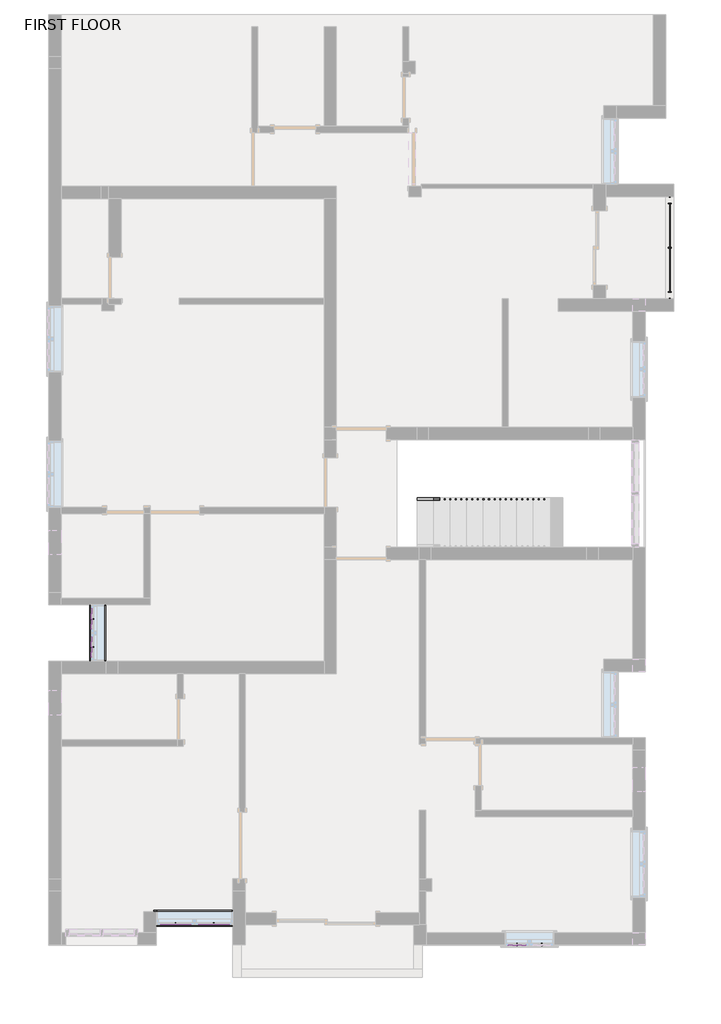
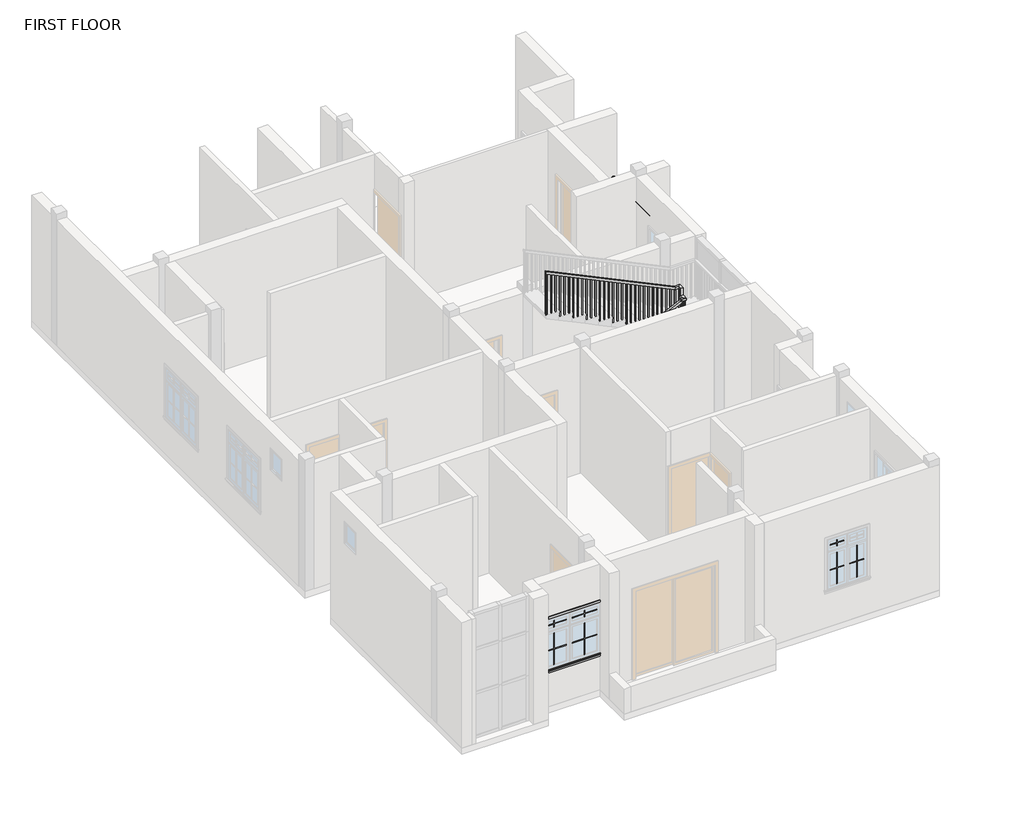
# One storey, part 5 of 6: 15 proxies, 2 railings.
"""IFC4 building model written with IfcOpenShell, lengths in millimetres."""

from ifc_helpers import new_model, si_unit, point, frame, origin, place, context, project, spatial, polyline, ellipse_curve, trimmed, outline, extrude, faceted_brep, transform, mapped, element, save
from ifc_brep_helpers import plane_surface, extruded_surface, advanced_brep
from components import muntin_pattern_2x2_muntin_pattern_2x2_a154cbfa, muntin_pattern_2x2_muntin_pattern_2x2_fbb866f2, muntin_pattern_2x2_muntin_pattern_2x2_1a5162a2, muntin_pattern_2x2_muntin_pattern_2x2_4af9dbf3, muntin_pattern_2x2_muntin_pattern_2x2_972acb6d, muntin_pattern_2x2_muntin_pattern_2x2_4879a4f3, muntin_pattern_2x2_muntin_pattern_2x2_d1c6e638, muntin_pattern_2x2_muntin_pattern_2x2_37b95fb2, muntin_pattern_2x2_muntin_pattern_2x2_604ffb00, trim_window_exterior_flat_with_sill_cb7cc766, trim_window_exterior_flat_with_sill_29d7a895, trim_window_interior_flat_picture_frame_9050e5f4, trim_window_interior_flat_picture_frame_56711e78

model = new_model("IFC4")

# Units and contexts
model_context = context("Model", 3, world=origin())
ifc_project = project(units=[si_unit("LENGTHUNIT", "METRE", prefix="MILLI")], contexts=[model_context])

# Site, building, storey
site = spatial("IfcSite", under=ifc_project)
building = spatial("IfcBuilding", under=site)
storey = spatial("IfcBuildingStorey", under=building, Name="FIRST FLOOR", Elevation=3200.4)

# Proxies
placement = place(None, origin())
muntin_pattern_2x2_muntin_pattern_2x2_shape = muntin_pattern_2x2_muntin_pattern_2x2_a154cbfa(model_context)
element("IfcBuildingElementProxy", 1, Name="Muntin Pattern_2x2 : Muntin Pattern_2x2", ObjectType="Muntin Pattern_2x2 : Muntin Pattern_2x2", at=placement, inside=storey, context=model_context, shape_type="MappedRepresentation", body=[
    mapped(muntin_pattern_2x2_muntin_pattern_2x2_shape, transform((-3731.5990981, -7428.8962413, 4184.65), x_axis=(-1.0, 0.0, 0.0), y_axis=(0.0, -1.0, 0.0), z_axis=(0.0, 0.0, 1.0))),
])
muntin_pattern_2x2_muntin_pattern_2x2_2_shape = muntin_pattern_2x2_muntin_pattern_2x2_fbb866f2(model_context)
element("IfcBuildingElementProxy", 2, Name="Muntin Pattern_2x2 : Muntin Pattern_2x2", ObjectType="Muntin Pattern_2x2 : Muntin Pattern_2x2", at=placement, inside=storey, context=model_context, shape_type="MappedRepresentation", body=[
    mapped(muntin_pattern_2x2_muntin_pattern_2x2_2_shape, transform((-4433.2740981, -7428.8962413, 4184.65), x_axis=(1.0, 0.0, 0.0), y_axis=(0.0, 1.0, 0.0), z_axis=(0.0, 0.0, 1.0))),
])
muntin_pattern_2x2_muntin_pattern_2x2_3_shape = muntin_pattern_2x2_muntin_pattern_2x2_1a5162a2(model_context)
element("IfcBuildingElementProxy", 3, Name="Muntin Pattern_2x2 : Muntin Pattern_2x2", ObjectType="Muntin Pattern_2x2 : Muntin Pattern_2x2", at=placement, inside=storey, context=model_context, shape_type="MappedRepresentation", body=[
    mapped(muntin_pattern_2x2_muntin_pattern_2x2_3_shape, transform((-4433.2740981, -7428.8962413, 5099.05), x_axis=(1.0, 0.0, 0.0), y_axis=(0.0, 1.0, 0.0), z_axis=(0.0, 0.0, 1.0))),
])
element("IfcBuildingElementProxy", 4, Name="Muntin Pattern_2x2 : Muntin Pattern_2x2", ObjectType="Muntin Pattern_2x2 : Muntin Pattern_2x2", at=placement, inside=storey, context=model_context, shape_type="MappedRepresentation", body=[
    mapped(muntin_pattern_2x2_muntin_pattern_2x2_3_shape, transform((-3731.5990981, -7428.8962413, 5099.05), x_axis=(1.0, 0.0, 0.0), y_axis=(0.0, 1.0, 0.0), z_axis=(0.0, 0.0, 1.0))),
])
muntin_pattern_2x2_muntin_pattern_2x2_4_shape = muntin_pattern_2x2_muntin_pattern_2x2_4af9dbf3(model_context)
element("IfcBuildingElementProxy", 5, Name="Muntin Pattern_2x2 : Muntin Pattern_2x2", ObjectType="Muntin Pattern_2x2 : Muntin Pattern_2x2", at=placement, inside=storey, context=model_context, shape_type="MappedRepresentation", body=[
    mapped(muntin_pattern_2x2_muntin_pattern_2x2_4_shape, transform((-5964.7636947, -2337.7837413, 4184.65), x_axis=(0.0, 1.0, 0.0), y_axis=(-1.0, 0.0, 0.0), z_axis=(0.0, 0.0, 1.0))),
])
muntin_pattern_2x2_muntin_pattern_2x2_5_shape = muntin_pattern_2x2_muntin_pattern_2x2_972acb6d(model_context)
element("IfcBuildingElementProxy", 6, Name="Muntin Pattern_2x2 : Muntin Pattern_2x2", ObjectType="Muntin Pattern_2x2 : Muntin Pattern_2x2", at=placement, inside=storey, context=model_context, shape_type="MappedRepresentation", body=[
    mapped(muntin_pattern_2x2_muntin_pattern_2x2_5_shape, transform((-5964.7636947, -1820.2587413, 4184.65), x_axis=(0.0, -1.0, 0.0), y_axis=(1.0, 0.0, 0.0), z_axis=(0.0, 0.0, 1.0))),
])
muntin_pattern_2x2_muntin_pattern_2x2_6_shape = muntin_pattern_2x2_muntin_pattern_2x2_4879a4f3(model_context)
element("IfcBuildingElementProxy", 7, Name="Muntin Pattern_2x2 : Muntin Pattern_2x2", ObjectType="Muntin Pattern_2x2 : Muntin Pattern_2x2", at=placement, inside=storey, context=model_context, shape_type="MappedRepresentation", body=[
    mapped(muntin_pattern_2x2_muntin_pattern_2x2_6_shape, transform((-5964.7636947, -1820.2587413, 5099.05), x_axis=(0.0, -1.0, 0.0), y_axis=(1.0, 0.0, 0.0), z_axis=(0.0, 0.0, 1.0))),
])
element("IfcBuildingElementProxy", 8, Name="Muntin Pattern_2x2 : Muntin Pattern_2x2", ObjectType="Muntin Pattern_2x2 : Muntin Pattern_2x2", at=placement, inside=storey, context=model_context, shape_type="MappedRepresentation", body=[
    mapped(muntin_pattern_2x2_muntin_pattern_2x2_6_shape, transform((-5964.7636947, -2337.7837413, 5099.05), x_axis=(0.0, -1.0, 0.0), y_axis=(1.0, 0.0, 0.0), z_axis=(0.0, 0.0, 1.0))),
])
muntin_pattern_2x2_muntin_pattern_2x2_7_shape = muntin_pattern_2x2_muntin_pattern_2x2_d1c6e638(model_context)
element("IfcBuildingElementProxy", 9, Name="Muntin Pattern_2x2 : Muntin Pattern_2x2", ObjectType="Muntin Pattern_2x2 : Muntin Pattern_2x2", at=placement, inside=storey, context=model_context, shape_type="MappedRepresentation", body=[
    mapped(muntin_pattern_2x2_muntin_pattern_2x2_7_shape, transform((2304.0759019, -7809.8962413, 4184.65), x_axis=(-1.0, 0.0, 0.0), y_axis=(0.0, -1.0, 0.0), z_axis=(0.0, 0.0, 1.0))),
])
muntin_pattern_2x2_muntin_pattern_2x2_8_shape = muntin_pattern_2x2_muntin_pattern_2x2_37b95fb2(model_context)
element("IfcBuildingElementProxy", 10, Name="Muntin Pattern_2x2 : Muntin Pattern_2x2", ObjectType="Muntin Pattern_2x2 : Muntin Pattern_2x2", at=placement, inside=storey, context=model_context, shape_type="MappedRepresentation", body=[
    mapped(muntin_pattern_2x2_muntin_pattern_2x2_8_shape, transform((1850.0509019, -7809.8962413, 4184.65), x_axis=(1.0, 0.0, 0.0), y_axis=(0.0, 1.0, 0.0), z_axis=(0.0, 0.0, 1.0))),
])
muntin_pattern_2x2_muntin_pattern_2x2_9_shape = muntin_pattern_2x2_muntin_pattern_2x2_604ffb00(model_context)
element("IfcBuildingElementProxy", 11, Name="Muntin Pattern_2x2 : Muntin Pattern_2x2", ObjectType="Muntin Pattern_2x2 : Muntin Pattern_2x2", at=placement, inside=storey, context=model_context, shape_type="MappedRepresentation", body=[
    mapped(muntin_pattern_2x2_muntin_pattern_2x2_9_shape, transform((1850.0509019, -7809.8962413, 5099.05), x_axis=(1.0, 0.0, 0.0), y_axis=(0.0, 1.0, 0.0), z_axis=(0.0, 0.0, 1.0))),
])
trim_window_exterior_flat_with_sill_shape = trim_window_exterior_flat_with_sill_cb7cc766(model_context)
element("IfcBuildingElementProxy", 12, Name="Trim-Window-Exterior-Flat : with Sill", ObjectType="Trim-Window-Exterior-Flat : with Sill", at=placement, inside=storey, context=model_context, shape_type="MappedRepresentation", body=[
    mapped(trim_window_exterior_flat_with_sill_shape, transform((-4082.4365981, -7438.4212413, 5334.0), x_axis=(1.0, 0.0, 0.0), y_axis=(0.0, 0.0, 1.0), z_axis=(0.0, -1.0, 0.0))),
])
trim_window_exterior_flat_with_sill_2_shape = trim_window_exterior_flat_with_sill_29d7a895(model_context)
element("IfcBuildingElementProxy", 13, Name="Trim-Window-Exterior-Flat : with Sill", ObjectType="Trim-Window-Exterior-Flat : with Sill", at=placement, inside=storey, context=model_context, shape_type="MappedRepresentation", body=[
    mapped(trim_window_exterior_flat_with_sill_2_shape, transform((-5974.2886947, -2079.0212413, 5334.0), x_axis=(0.0, -1.0, 0.0), y_axis=(0.0, 0.0, 1.0), z_axis=(-1.0, 0.0, 0.0))),
])
trim_window_interior_flat_picture_frame_shape = trim_window_interior_flat_picture_frame_9050e5f4(model_context)
element("IfcBuildingElementProxy", 14, Name="Trim-Window-Interior-Flat : Picture Frame", ObjectType="Trim-Window-Interior-Flat : Picture Frame", at=placement, inside=storey, context=model_context, shape_type="MappedRepresentation", body=[
    mapped(trim_window_interior_flat_picture_frame_shape, transform((-4082.4365981, -7209.8212413, 5334.0), x_axis=(-1.0, 0.0, 0.0), y_axis=(0.0, 0.0, 1.0), z_axis=(0.0, 1.0, 0.0))),
])
trim_window_interior_flat_picture_frame_2_shape = trim_window_interior_flat_picture_frame_56711e78(model_context)
element("IfcBuildingElementProxy", 15, Name="Trim-Window-Interior-Flat : Picture Frame", ObjectType="Trim-Window-Interior-Flat : Picture Frame", at=placement, inside=storey, context=model_context, shape_type="MappedRepresentation", body=[
    mapped(trim_window_interior_flat_picture_frame_2_shape, transform((-5745.6886947, -2079.0212413, 5334.0), x_axis=(0.0, 1.0, 0.0), y_axis=(0.0, 0.0, 1.0), z_axis=(1.0, 0.0, 0.0))),
])

# Railings
element("IfcRailing", 16, ObjectType="Glass Panel - Bottom Fill", at=placement, inside=storey, context=model_context, shape_type="SolidModel", body=[
    advanced_brep(
    [(4699.6134019, 5947.3787587, 4724.4), (4623.4134019, 5947.3787587, 4724.4), (4699.6134019, 4067.7787587, 4724.4), (4623.4134019, 4067.7787587, 4724.4)],
    [
        (0, 1, ellipse_curve(frame((4661.5134019, 5947.3787587, 4724.4), z_axis=(0.0, 1.0, 0.0), x_axis=(-1.0, 0.0, 0.0)), 38.1, 28.575)),
        (1, 0, ellipse_curve(frame((4661.5134019, 5947.3787587, 4724.4), z_axis=(0.0, 1.0, 0.0), x_axis=(-1.0, 0.0, 0.0)), 38.1, 28.575)),
        (2, 3, ellipse_curve(frame((4661.5134019, 4067.7787587, 4724.4), z_axis=(0.0, -1.0, 0.0), x_axis=(-1.0, 0.0, 0.0)), 38.1, 28.575)),
        (3, 2, ellipse_curve(frame((4661.5134019, 4067.7787587, 4724.4), z_axis=(0.0, -1.0, 0.0), x_axis=(-1.0, 0.0, 0.0)), 38.1, 28.575)),
        (0, 2),
        (3, 1),
    ],
    [
        plane_surface(frame((4661.5134019, 5947.3787587, 4724.4), z_axis=(0.0, 1.0, 0.0), x_axis=(0.0, 0.0, -1.0))),
        plane_surface(frame((4661.5134019, 4067.7787587, 4724.4), z_axis=(0.0, -1.0, 0.0), x_axis=(0.0, 0.0, -1.0))),
        extruded_surface(trimmed(ellipse_curve(frame((4661.5134019, 4067.7787587, 4724.4), z_axis=(0.0, 1.0, 0.0), x_axis=(-1.0, 0.0, 0.0)), 38.1, 28.575), [point((4699.6134019, 4067.7787587, 4724.4))], [point((4623.4134019, 4067.7787587, 4724.4))], True, "CARTESIAN"), (0.0, 1879.6, 0.0), 1879.6),
        extruded_surface(trimmed(ellipse_curve(frame((4661.5134019, 4067.7787587, 4724.4), z_axis=(0.0, 1.0, 0.0), x_axis=(-1.0, 0.0, 0.0)), 38.1, 28.575), [point((4623.4134019, 4067.7787587, 4724.4))], [point((4699.6134019, 4067.7787587, 4724.4))], True, "CARTESIAN"), (0.0, 1879.6, 0.0), 1879.6),
    ],
    [
        (0, [[1, 2]]),
        (1, [[3, 4]]),
        (2, [[-1, 5, -4, 6]]),
        (3, [[-2, -6, -3, -5]]),
    ],
),
    extrude(outline(polyline([(4648.8134019, 5947.3787587), (4674.2134019, 5947.3787587), (4674.2134019, 4067.7787587), (4648.8134019, 4067.7787587), (4648.8134019, 5947.3787587)])), frame((0.0, 0.0, 4610.1), z_axis=(0.0, 0.0, 1.0), x_axis=(1.0, 0.0, 0.0)), (0.0, 0.0, 1.0), 25.4),
    extrude(outline(polyline([(4648.8134019, 5947.3787587), (4674.2134019, 5947.3787587), (4674.2134019, 4067.7787587), (4648.8134019, 4067.7787587), (4648.8134019, 5947.3787587)])), frame((0.0, 0.0, 4508.5), z_axis=(0.0, 0.0, 1.0), x_axis=(1.0, 0.0, 0.0)), (0.0, 0.0, 1.0), 25.4),
    extrude(outline(polyline([(4636.1134019, 4201.1287587), (4686.9134019, 4201.1287587), (4686.9134019, 4188.4287587), (4636.1134019, 4188.4287587), (4636.1134019, 4201.1287587)])), frame((0.0, 0.0, 3810.0), z_axis=(0.0, 0.0, 1.0), x_axis=(1.0, 0.0, 0.0)), (0.0, 0.0, 1.0), 885.825),
    extrude(outline(polyline([(4668.0485589, 5007.5787587), (4668.0485589, 4194.7787587), (4661.6985589, 4194.7787587), (4661.6985589, 5007.5787587), (4668.0485589, 5007.5787587)])), frame((0.0, 0.0, 3911.6), z_axis=(0.0, 0.0, 1.0), x_axis=(1.0, 0.0, 0.0)), (0.0, 0.0, 1.0), 596.9),
    extrude(outline(polyline([(4636.1134019, 5013.9287587), (4686.9134019, 5013.9287587), (4686.9134019, 5001.2287587), (4636.1134019, 5001.2287587), (4636.1134019, 5013.9287587)])), frame((0.0, 0.0, 3810.0), z_axis=(0.0, 0.0, 1.0), x_axis=(1.0, 0.0, 0.0)), (0.0, 0.0, 1.0), 885.825),
    extrude(outline(polyline([(4668.0485589, 5820.3787587), (4668.0485589, 5007.5787587), (4661.6985589, 5007.5787587), (4661.6985589, 5820.3787587), (4668.0485589, 5820.3787587)])), frame((0.0, 0.0, 3911.6), z_axis=(0.0, 0.0, 1.0), x_axis=(1.0, 0.0, 0.0)), (0.0, 0.0, 1.0), 596.9),
    extrude(outline(polyline([(4636.1134019, 5826.7287587), (4686.9134019, 5826.7287587), (4686.9134019, 5814.0287587), (4636.1134019, 5814.0287587), (4636.1134019, 5826.7287587)])), frame((0.0, 0.0, 3810.0), z_axis=(0.0, 0.0, 1.0), x_axis=(1.0, 0.0, 0.0)), (0.0, 0.0, 1.0), 885.825),
    extrude(outline(polyline([(4651.9884019, 4080.4787587), (4671.0384019, 4080.4787587), (4671.0384019, 4061.4287587), (4651.9884019, 4061.4287587), (4651.9884019, 4080.4787587)])), frame((0.0, 0.0, 3810.0), z_axis=(0.0, 0.0, 1.0), x_axis=(1.0, 0.0, 0.0)), (0.0, 0.0, 1.0), 885.825),
    extrude(outline(polyline([(4651.9884019, 5953.7287587), (4671.0384019, 5953.7287587), (4671.0384019, 5934.6787587), (4651.9884019, 5934.6787587), (4651.9884019, 5953.7287587)])), frame((0.0, 0.0, 3810.0), z_axis=(0.0, 0.0, 1.0), x_axis=(1.0, 0.0, 0.0)), (0.0, 0.0, 1.0), 885.825),
])
element("IfcRailing", 17, ObjectType="Handrail - Rectangular", at=placement, inside=storey, context=model_context, shape_type="SolidModel", body=[
    faceted_brep([(13.3134019, 410.1787587, 4260.2727273), (13.3134019, 410.1787587, 4203.9834559), (13.3134019, 359.3787587, 4203.9834559), (13.3134019, 359.3787587, 4260.2727273), (2985.1134019, 410.1787587, 5678.6318182), (3035.9134019, 410.1787587, 5646.5880014), (3035.9134019, 359.3787587, 5646.5880014), (2985.1134019, 359.3787587, 5678.6318182), (2985.1134019, 410.1787587, 5715.0), (3035.9134019, 410.1787587, 5664.2), (3035.9134019, 359.3787587, 5664.2), (2985.1134019, 359.3787587, 5715.0), (3061.3134019, 410.1787587, 5715.0), (3061.3134019, 410.1787587, 5664.2), (3112.1134019, 359.3787587, 5664.2), (3112.1134019, 359.3787587, 5715.0), (3061.3134019, 486.3787587, 5715.0), (3061.3134019, 537.1787587, 5664.2), (3112.1134019, 537.1787587, 5664.2), (3112.1134019, 486.3787587, 5715.0), (3061.3134019, 486.3787587, 5896.8409091), (3061.3134019, 537.1787587, 5846.0409091), (3112.1134019, 537.1787587, 5846.0409091), (3112.1134019, 486.3787587, 5896.8409091), (3061.3134019, 562.5787587, 5896.8409091), (3061.3134019, 562.5787587, 5846.0409091), (3112.1134019, 613.3787587, 5846.0409091), (3112.1134019, 613.3787587, 5896.8409091), (2985.1134019, 562.5787587, 5896.8409091), (2973.6120715, 562.5787587, 5846.0409091), (2973.6120715, 613.3787587, 5846.0409091), (2985.1134019, 613.3787587, 5896.8409091), (13.3134019, 562.5787587, 7315.2), (13.3134019, 613.3787587, 7315.2), (13.3134019, 613.3787587, 7258.9107287), (13.3134019, 562.5787587, 7258.9107287)], [[[0, 1, 2, 3]], [[1, 0, 4, 5]], [[2, 1, 5, 6]], [[3, 2, 6, 7]], [[0, 3, 7, 4]], [[5, 4, 8, 9]], [[6, 5, 9, 10]], [[7, 6, 10, 11]], [[4, 7, 11, 8]], [[9, 8, 12, 13]], [[10, 9, 13, 14]], [[11, 10, 14, 15]], [[8, 11, 15, 12]], [[13, 12, 16, 17]], [[14, 13, 17, 18]], [[15, 14, 18, 19]], [[12, 15, 19, 16]], [[17, 16, 20, 21]], [[18, 17, 21, 22]], [[19, 18, 22, 23]], [[16, 19, 23, 20]], [[21, 20, 24, 25]], [[22, 21, 25, 26]], [[23, 22, 26, 27]], [[20, 23, 27, 24]], [[25, 24, 28, 29]], [[26, 25, 29, 30]], [[27, 26, 30, 31]], [[24, 27, 31, 28]], [[32, 33, 34, 35]], [[29, 28, 32, 35]], [[30, 29, 35, 34]], [[31, 30, 34, 33]], [[28, 31, 33, 32]]]),
    extrude(outline(polyline([(7251.3340241, 29.1884019), (6255.3272727, 29.1884019), (6255.3272727, 48.2384019), (7242.2419787, 48.2384019), (7251.3340241, 29.1884019)])), frame((0.0, 578.4537587, 0.0), z_axis=(0.0, 1.0, 0.0), x_axis=(0.0, 0.0, 1.0)), (0.0, 0.0, 1.0), 19.05),
    extrude(outline(polyline([(7202.843115, 130.7884019), (6255.3272727, 130.7884019), (6255.3272727, 149.8384019), (7193.7510696, 149.8384019), (7202.843115, 130.7884019)])), frame((0.0, 578.4537587, 0.0), z_axis=(0.0, 1.0, 0.0), x_axis=(0.0, 0.0, 1.0)), (0.0, 0.0, 1.0), 19.05),
    extrude(outline(polyline([(7154.3522059, 232.3884019), (6255.3272727, 232.3884019), (6255.3272727, 251.4384019), (7145.2601605, 251.4384019), (7154.3522059, 232.3884019)])), frame((0.0, 578.4537587, 0.0), z_axis=(0.0, 1.0, 0.0), x_axis=(0.0, 0.0, 1.0)), (0.0, 0.0, 1.0), 19.05),
    extrude(outline(polyline([(7105.8612969, 333.9884019), (6109.8545455, 333.9884019), (6109.8545455, 353.0384019), (7096.7692514, 353.0384019), (7105.8612969, 333.9884019)])), frame((0.0, 578.4537587, 0.0), z_axis=(0.0, 1.0, 0.0), x_axis=(0.0, 0.0, 1.0)), (0.0, 0.0, 1.0), 19.05),
    extrude(outline(polyline([(7057.3703878, 435.5884019), (6109.8545455, 435.5884019), (6109.8545455, 454.6384019), (7048.2783423, 454.6384019), (7057.3703878, 435.5884019)])), frame((0.0, 578.4537587, 0.0), z_axis=(0.0, 1.0, 0.0), x_axis=(0.0, 0.0, 1.0)), (0.0, 0.0, 1.0), 19.05),
    extrude(outline(polyline([(7008.8794787, 537.1884019), (6109.8545455, 537.1884019), (6109.8545455, 556.2384019), (6999.7874332, 556.2384019), (7008.8794787, 537.1884019)])), frame((0.0, 578.4537587, 0.0), z_axis=(0.0, 1.0, 0.0), x_axis=(0.0, 0.0, 1.0)), (0.0, 0.0, 1.0), 19.05),
    extrude(outline(polyline([(6960.3885696, 638.7884019), (5964.3818182, 638.7884019), (5964.3818182, 657.8384019), (6951.2965241, 657.8384019), (6960.3885696, 638.7884019)])), frame((0.0, 578.4537587, 0.0), z_axis=(0.0, 1.0, 0.0), x_axis=(0.0, 0.0, 1.0)), (0.0, 0.0, 1.0), 19.05),
    extrude(outline(polyline([(6911.8976605, 740.3884019), (5964.3818182, 740.3884019), (5964.3818182, 759.4384019), (6902.805615, 759.4384019), (6911.8976605, 740.3884019)])), frame((0.0, 578.4537587, 0.0), z_axis=(0.0, 1.0, 0.0), x_axis=(0.0, 0.0, 1.0)), (0.0, 0.0, 1.0), 19.05),
    extrude(outline(polyline([(6863.4067514, 841.9884019), (5964.3818182, 841.9884019), (5964.3818182, 861.0384019), (6854.3147059, 861.0384019), (6863.4067514, 841.9884019)])), frame((0.0, 578.4537587, 0.0), z_axis=(0.0, 1.0, 0.0), x_axis=(0.0, 0.0, 1.0)), (0.0, 0.0, 1.0), 19.05),
    extrude(outline(polyline([(6814.9158423, 943.5884019), (5818.9090909, 943.5884019), (5818.9090909, 962.6384019), (6805.8237969, 962.6384019), (6814.9158423, 943.5884019)])), frame((0.0, 578.4537587, 0.0), z_axis=(0.0, 1.0, 0.0), x_axis=(0.0, 0.0, 1.0)), (0.0, 0.0, 1.0), 19.05),
    extrude(outline(polyline([(6766.4249332, 1045.1884019), (5818.9090909, 1045.1884019), (5818.9090909, 1064.2384019), (6757.3328878, 1064.2384019), (6766.4249332, 1045.1884019)])), frame((0.0, 578.4537587, 0.0), z_axis=(0.0, 1.0, 0.0), x_axis=(0.0, 0.0, 1.0)), (0.0, 0.0, 1.0), 19.05),
    extrude(outline(polyline([(6717.9340241, 1146.7884019), (5818.9090909, 1146.7884019), (5818.9090909, 1165.8384019), (6708.8419787, 1165.8384019), (6717.9340241, 1146.7884019)])), frame((0.0, 578.4537587, 0.0), z_axis=(0.0, 1.0, 0.0), x_axis=(0.0, 0.0, 1.0)), (0.0, 0.0, 1.0), 19.05),
    extrude(outline(polyline([(6669.443115, 1248.3884019), (5673.4363636, 1248.3884019), (5673.4363636, 1267.4384019), (6660.3510696, 1267.4384019), (6669.443115, 1248.3884019)])), frame((0.0, 578.4537587, 0.0), z_axis=(0.0, 1.0, 0.0), x_axis=(0.0, 0.0, 1.0)), (0.0, 0.0, 1.0), 19.05),
    extrude(outline(polyline([(6620.9522059, 1349.9884019), (5673.4363636, 1349.9884019), (5673.4363636, 1369.0384019), (6611.8601605, 1369.0384019), (6620.9522059, 1349.9884019)])), frame((0.0, 578.4537587, 0.0), z_axis=(0.0, 1.0, 0.0), x_axis=(0.0, 0.0, 1.0)), (0.0, 0.0, 1.0), 19.05),
    extrude(outline(polyline([(6572.4612969, 1451.5884019), (5673.4363636, 1451.5884019), (5673.4363636, 1470.6384019), (6563.3692514, 1470.6384019), (6572.4612969, 1451.5884019)])), frame((0.0, 578.4537587, 0.0), z_axis=(0.0, 1.0, 0.0), x_axis=(0.0, 0.0, 1.0)), (0.0, 0.0, 1.0), 19.05),
    extrude(outline(polyline([(6523.9703878, 1553.1884019), (5527.9636364, 1553.1884019), (5527.9636364, 1572.2384019), (6514.8783423, 1572.2384019), (6523.9703878, 1553.1884019)])), frame((0.0, 578.4537587, 0.0), z_axis=(0.0, 1.0, 0.0), x_axis=(0.0, 0.0, 1.0)), (0.0, 0.0, 1.0), 19.05),
    extrude(outline(polyline([(6475.4794787, 1654.7884019), (5527.9636364, 1654.7884019), (5527.9636364, 1673.8384019), (6466.3874332, 1673.8384019), (6475.4794787, 1654.7884019)])), frame((0.0, 578.4537587, 0.0), z_axis=(0.0, 1.0, 0.0), x_axis=(0.0, 0.0, 1.0)), (0.0, 0.0, 1.0), 19.05),
    extrude(outline(polyline([(6426.9885696, 1756.3884019), (5527.9636364, 1756.3884019), (5527.9636364, 1775.4384019), (6417.8965241, 1775.4384019), (6426.9885696, 1756.3884019)])), frame((0.0, 578.4537587, 0.0), z_axis=(0.0, 1.0, 0.0), x_axis=(0.0, 0.0, 1.0)), (0.0, 0.0, 1.0), 19.05),
    extrude(outline(polyline([(6378.4976605, 1857.9884019), (5382.4909091, 1857.9884019), (5382.4909091, 1877.0384019), (6369.405615, 1877.0384019), (6378.4976605, 1857.9884019)])), frame((0.0, 578.4537587, 0.0), z_axis=(0.0, 1.0, 0.0), x_axis=(0.0, 0.0, 1.0)), (0.0, 0.0, 1.0), 19.05),
    extrude(outline(polyline([(6330.0067514, 1959.5884019), (5382.4909091, 1959.5884019), (5382.4909091, 1978.6384019), (6320.9147059, 1978.6384019), (6330.0067514, 1959.5884019)])), frame((0.0, 578.4537587, 0.0), z_axis=(0.0, 1.0, 0.0), x_axis=(0.0, 0.0, 1.0)), (0.0, 0.0, 1.0), 19.05),
    extrude(outline(polyline([(6281.5158423, 2061.1884019), (5382.4909091, 2061.1884019), (5382.4909091, 2080.2384019), (6272.4237969, 2080.2384019), (6281.5158423, 2061.1884019)])), frame((0.0, 578.4537587, 0.0), z_axis=(0.0, 1.0, 0.0), x_axis=(0.0, 0.0, 1.0)), (0.0, 0.0, 1.0), 19.05),
    extrude(outline(polyline([(6233.0249332, 2162.7884019), (5237.0181818, 2162.7884019), (5237.0181818, 2181.8384019), (6223.9328878, 2181.8384019), (6233.0249332, 2162.7884019)])), frame((0.0, 578.4537587, 0.0), z_axis=(0.0, 1.0, 0.0), x_axis=(0.0, 0.0, 1.0)), (0.0, 0.0, 1.0), 19.05),
    extrude(outline(polyline([(6184.5340241, 2264.3884019), (5237.0181818, 2264.3884019), (5237.0181818, 2283.4384019), (6175.4419787, 2283.4384019), (6184.5340241, 2264.3884019)])), frame((0.0, 578.4537587, 0.0), z_axis=(0.0, 1.0, 0.0), x_axis=(0.0, 0.0, 1.0)), (0.0, 0.0, 1.0), 19.05),
    extrude(outline(polyline([(6136.043115, 2365.9884019), (5237.0181818, 2365.9884019), (5237.0181818, 2385.0384019), (6126.9510696, 2385.0384019), (6136.043115, 2365.9884019)])), frame((0.0, 578.4537587, 0.0), z_axis=(0.0, 1.0, 0.0), x_axis=(0.0, 0.0, 1.0)), (0.0, 0.0, 1.0), 19.05),
    extrude(outline(polyline([(6087.5522059, 2467.5884019), (5091.5454545, 2467.5884019), (5091.5454545, 2486.6384019), (6078.4601605, 2486.6384019), (6087.5522059, 2467.5884019)])), frame((0.0, 578.4537587, 0.0), z_axis=(0.0, 1.0, 0.0), x_axis=(0.0, 0.0, 1.0)), (0.0, 0.0, 1.0), 19.05),
    extrude(outline(polyline([(6039.0612969, 2569.1884019), (5091.5454545, 2569.1884019), (5091.5454545, 2588.2384019), (6029.9692514, 2588.2384019), (6039.0612969, 2569.1884019)])), frame((0.0, 578.4537587, 0.0), z_axis=(0.0, 1.0, 0.0), x_axis=(0.0, 0.0, 1.0)), (0.0, 0.0, 1.0), 19.05),
    extrude(outline(polyline([(5990.5703878, 2670.7884019), (5091.5454545, 2670.7884019), (5091.5454545, 2689.8384019), (5981.4783423, 2689.8384019), (5990.5703878, 2670.7884019)])), frame((0.0, 578.4537587, 0.0), z_axis=(0.0, 1.0, 0.0), x_axis=(0.0, 0.0, 1.0)), (0.0, 0.0, 1.0), 19.05),
    extrude(outline(polyline([(5942.0794787, 2772.3884019), (4946.0727273, 2772.3884019), (4946.0727273, 2791.4384019), (5932.9874332, 2791.4384019), (5942.0794787, 2772.3884019)])), frame((0.0, 578.4537587, 0.0), z_axis=(0.0, 1.0, 0.0), x_axis=(0.0, 0.0, 1.0)), (0.0, 0.0, 1.0), 19.05),
    extrude(outline(polyline([(5893.5885696, 2873.9884019), (4946.0727273, 2873.9884019), (4946.0727273, 2893.0384019), (5884.4965241, 2893.0384019), (5893.5885696, 2873.9884019)])), frame((0.0, 578.4537587, 0.0), z_axis=(0.0, 1.0, 0.0), x_axis=(0.0, 0.0, 1.0)), (0.0, 0.0, 1.0), 19.05),
    extrude(outline(polyline([(5845.0976605, 2975.5884019), (4946.0727273, 2975.5884019), (4946.0727273, 2994.6384019), (5836.005615, 2994.6384019), (5845.0976605, 2975.5884019)])), frame((0.0, 578.4537587, 0.0), z_axis=(0.0, 1.0, 0.0), x_axis=(0.0, 0.0, 1.0)), (0.0, 0.0, 1.0), 19.05),
    extrude(outline(polyline([(3077.1884019, 476.8537587), (3077.1884019, 495.9037587), (3096.2384019, 495.9037587), (3096.2384019, 476.8537587), (3077.1884019, 476.8537587)])), frame((0.0, 0.0, 4800.6), z_axis=(0.0, 0.0, 1.0), x_axis=(1.0, 0.0, 0.0)), (0.0, 0.0, 1.0), 863.6),
    extrude(outline(polyline([(3051.7884019, 394.3037587), (3070.8384019, 394.3037587), (3070.8384019, 375.2537587), (3051.7884019, 375.2537587), (3051.7884019, 394.3037587)])), frame((0.0, 0.0, 4800.6), z_axis=(0.0, 0.0, 1.0), x_axis=(1.0, 0.0, 0.0)), (0.0, 0.0, 1.0), 863.6),
    extrude(outline(polyline([(5605.6737969, 2950.1884019), (4655.1272727, 2950.1884019), (4655.1272727, 2969.2384019), (5614.7658423, 2969.2384019), (5605.6737969, 2950.1884019)])), frame((0.0, 375.2537587, 0.0), z_axis=(0.0, 1.0, 0.0), x_axis=(0.0, 0.0, 1.0)), (0.0, 0.0, 1.0), 19.05),
    extrude(outline(polyline([(5557.1828878, 2848.5884019), (4655.1272727, 2848.5884019), (4655.1272727, 2867.6384019), (5566.2749332, 2867.6384019), (5557.1828878, 2848.5884019)])), frame((0.0, 375.2537587, 0.0), z_axis=(0.0, 1.0, 0.0), x_axis=(0.0, 0.0, 1.0)), (0.0, 0.0, 1.0), 19.05),
    extrude(outline(polyline([(5508.6919787, 2746.9884019), (4655.1272727, 2746.9884019), (4655.1272727, 2766.0384019), (5517.7840241, 2766.0384019), (5508.6919787, 2746.9884019)])), frame((0.0, 375.2537587, 0.0), z_axis=(0.0, 1.0, 0.0), x_axis=(0.0, 0.0, 1.0)), (0.0, 0.0, 1.0), 19.05),
    extrude(outline(polyline([(5460.2010696, 2645.3884019), (4509.6545455, 2645.3884019), (4509.6545455, 2664.4384019), (5469.293115, 2664.4384019), (5460.2010696, 2645.3884019)])), frame((0.0, 375.2537587, 0.0), z_axis=(0.0, 1.0, 0.0), x_axis=(0.0, 0.0, 1.0)), (0.0, 0.0, 1.0), 19.05),
    extrude(outline(polyline([(5411.7101605, 2543.7884019), (4509.6545455, 2543.7884019), (4509.6545455, 2562.8384019), (5420.8022059, 2562.8384019), (5411.7101605, 2543.7884019)])), frame((0.0, 375.2537587, 0.0), z_axis=(0.0, 1.0, 0.0), x_axis=(0.0, 0.0, 1.0)), (0.0, 0.0, 1.0), 19.05),
    extrude(outline(polyline([(5363.2192514, 2442.1884019), (4509.6545455, 2442.1884019), (4509.6545455, 2461.2384019), (5372.3112969, 2461.2384019), (5363.2192514, 2442.1884019)])), frame((0.0, 375.2537587, 0.0), z_axis=(0.0, 1.0, 0.0), x_axis=(0.0, 0.0, 1.0)), (0.0, 0.0, 1.0), 19.05),
    extrude(outline(polyline([(5314.7283423, 2340.5884019), (4364.1818182, 2340.5884019), (4364.1818182, 2359.6384019), (5323.8203878, 2359.6384019), (5314.7283423, 2340.5884019)])), frame((0.0, 375.2537587, 0.0), z_axis=(0.0, 1.0, 0.0), x_axis=(0.0, 0.0, 1.0)), (0.0, 0.0, 1.0), 19.05),
    extrude(outline(polyline([(5266.2374332, 2238.9884019), (4364.1818182, 2238.9884019), (4364.1818182, 2258.0384019), (5275.3294787, 2258.0384019), (5266.2374332, 2238.9884019)])), frame((0.0, 375.2537587, 0.0), z_axis=(0.0, 1.0, 0.0), x_axis=(0.0, 0.0, 1.0)), (0.0, 0.0, 1.0), 19.05),
    extrude(outline(polyline([(5217.7465241, 2137.3884019), (4364.1818182, 2137.3884019), (4364.1818182, 2156.4384019), (5226.8385696, 2156.4384019), (5217.7465241, 2137.3884019)])), frame((0.0, 375.2537587, 0.0), z_axis=(0.0, 1.0, 0.0), x_axis=(0.0, 0.0, 1.0)), (0.0, 0.0, 1.0), 19.05),
    extrude(outline(polyline([(5169.255615, 2035.7884019), (4218.7090909, 2035.7884019), (4218.7090909, 2054.8384019), (5178.3476605, 2054.8384019), (5169.255615, 2035.7884019)])), frame((0.0, 375.2537587, 0.0), z_axis=(0.0, 1.0, 0.0), x_axis=(0.0, 0.0, 1.0)), (0.0, 0.0, 1.0), 19.05),
    extrude(outline(polyline([(5120.7647059, 1934.1884019), (4218.7090909, 1934.1884019), (4218.7090909, 1953.2384019), (5129.8567514, 1953.2384019), (5120.7647059, 1934.1884019)])), frame((0.0, 375.2537587, 0.0), z_axis=(0.0, 1.0, 0.0), x_axis=(0.0, 0.0, 1.0)), (0.0, 0.0, 1.0), 19.05),
    extrude(outline(polyline([(5072.2737969, 1832.5884019), (4218.7090909, 1832.5884019), (4218.7090909, 1851.6384019), (5081.3658423, 1851.6384019), (5072.2737969, 1832.5884019)])), frame((0.0, 375.2537587, 0.0), z_axis=(0.0, 1.0, 0.0), x_axis=(0.0, 0.0, 1.0)), (0.0, 0.0, 1.0), 19.05),
    extrude(outline(polyline([(5023.7828878, 1730.9884019), (4073.2363636, 1730.9884019), (4073.2363636, 1750.0384019), (5032.8749332, 1750.0384019), (5023.7828878, 1730.9884019)])), frame((0.0, 375.2537587, 0.0), z_axis=(0.0, 1.0, 0.0), x_axis=(0.0, 0.0, 1.0)), (0.0, 0.0, 1.0), 19.05),
    extrude(outline(polyline([(4975.2919787, 1629.3884019), (4073.2363636, 1629.3884019), (4073.2363636, 1648.4384019), (4984.3840241, 1648.4384019), (4975.2919787, 1629.3884019)])), frame((0.0, 375.2537587, 0.0), z_axis=(0.0, 1.0, 0.0), x_axis=(0.0, 0.0, 1.0)), (0.0, 0.0, 1.0), 19.05),
    extrude(outline(polyline([(4926.8010696, 1527.7884019), (4073.2363636, 1527.7884019), (4073.2363636, 1546.8384019), (4935.893115, 1546.8384019), (4926.8010696, 1527.7884019)])), frame((0.0, 375.2537587, 0.0), z_axis=(0.0, 1.0, 0.0), x_axis=(0.0, 0.0, 1.0)), (0.0, 0.0, 1.0), 19.05),
    extrude(outline(polyline([(4878.3101605, 1426.1884019), (3927.7636364, 1426.1884019), (3927.7636364, 1445.2384019), (4887.4022059, 1445.2384019), (4878.3101605, 1426.1884019)])), frame((0.0, 375.2537587, 0.0), z_axis=(0.0, 1.0, 0.0), x_axis=(0.0, 0.0, 1.0)), (0.0, 0.0, 1.0), 19.05),
    extrude(outline(polyline([(4829.8192514, 1324.5884019), (3927.7636364, 1324.5884019), (3927.7636364, 1343.6384019), (4838.9112969, 1343.6384019), (4829.8192514, 1324.5884019)])), frame((0.0, 375.2537587, 0.0), z_axis=(0.0, 1.0, 0.0), x_axis=(0.0, 0.0, 1.0)), (0.0, 0.0, 1.0), 19.05),
    extrude(outline(polyline([(4781.3283423, 1222.9884019), (3927.7636364, 1222.9884019), (3927.7636364, 1242.0384019), (4790.4203878, 1242.0384019), (4781.3283423, 1222.9884019)])), frame((0.0, 375.2537587, 0.0), z_axis=(0.0, 1.0, 0.0), x_axis=(0.0, 0.0, 1.0)), (0.0, 0.0, 1.0), 19.05),
    extrude(outline(polyline([(4732.8374332, 1121.3884019), (3782.2909091, 1121.3884019), (3782.2909091, 1140.4384019), (4741.9294787, 1140.4384019), (4732.8374332, 1121.3884019)])), frame((0.0, 375.2537587, 0.0), z_axis=(0.0, 1.0, 0.0), x_axis=(0.0, 0.0, 1.0)), (0.0, 0.0, 1.0), 19.05),
    extrude(outline(polyline([(4684.3465241, 1019.7884019), (3782.2909091, 1019.7884019), (3782.2909091, 1038.8384019), (4693.4385696, 1038.8384019), (4684.3465241, 1019.7884019)])), frame((0.0, 375.2537587, 0.0), z_axis=(0.0, 1.0, 0.0), x_axis=(0.0, 0.0, 1.0)), (0.0, 0.0, 1.0), 19.05),
    extrude(outline(polyline([(4635.855615, 918.1884019), (3782.2909091, 918.1884019), (3782.2909091, 937.2384019), (4644.9476605, 937.2384019), (4635.855615, 918.1884019)])), frame((0.0, 375.2537587, 0.0), z_axis=(0.0, 1.0, 0.0), x_axis=(0.0, 0.0, 1.0)), (0.0, 0.0, 1.0), 19.05),
    extrude(outline(polyline([(4587.3647059, 816.5884019), (3636.8181818, 816.5884019), (3636.8181818, 835.6384019), (4596.4567514, 835.6384019), (4587.3647059, 816.5884019)])), frame((0.0, 375.2537587, 0.0), z_axis=(0.0, 1.0, 0.0), x_axis=(0.0, 0.0, 1.0)), (0.0, 0.0, 1.0), 19.05),
    extrude(outline(polyline([(4538.8737969, 714.9884019), (3636.8181818, 714.9884019), (3636.8181818, 734.0384019), (4547.9658423, 734.0384019), (4538.8737969, 714.9884019)])), frame((0.0, 375.2537587, 0.0), z_axis=(0.0, 1.0, 0.0), x_axis=(0.0, 0.0, 1.0)), (0.0, 0.0, 1.0), 19.05),
    extrude(outline(polyline([(4490.3828878, 613.3884019), (3636.8181818, 613.3884019), (3636.8181818, 632.4384019), (4499.4749332, 632.4384019), (4490.3828878, 613.3884019)])), frame((0.0, 375.2537587, 0.0), z_axis=(0.0, 1.0, 0.0), x_axis=(0.0, 0.0, 1.0)), (0.0, 0.0, 1.0), 19.05),
    extrude(outline(polyline([(4441.8919787, 511.7884019), (3491.3454545, 511.7884019), (3491.3454545, 530.8384019), (4450.9840241, 530.8384019), (4441.8919787, 511.7884019)])), frame((0.0, 375.2537587, 0.0), z_axis=(0.0, 1.0, 0.0), x_axis=(0.0, 0.0, 1.0)), (0.0, 0.0, 1.0), 19.05),
    extrude(outline(polyline([(4393.4010696, 410.1884019), (3491.3454545, 410.1884019), (3491.3454545, 429.2384019), (4402.493115, 429.2384019), (4393.4010696, 410.1884019)])), frame((0.0, 375.2537587, 0.0), z_axis=(0.0, 1.0, 0.0), x_axis=(0.0, 0.0, 1.0)), (0.0, 0.0, 1.0), 19.05),
    extrude(outline(polyline([(4344.9101605, 308.5884019), (3491.3454545, 308.5884019), (3491.3454545, 327.6384019), (4354.0022059, 327.6384019), (4344.9101605, 308.5884019)])), frame((0.0, 375.2537587, 0.0), z_axis=(0.0, 1.0, 0.0), x_axis=(0.0, 0.0, 1.0)), (0.0, 0.0, 1.0), 19.05),
    extrude(outline(polyline([(4296.4192514, 206.9884019), (3345.8727273, 206.9884019), (3345.8727273, 226.0384019), (4305.5112969, 226.0384019), (4296.4192514, 206.9884019)])), frame((0.0, 375.2537587, 0.0), z_axis=(0.0, 1.0, 0.0), x_axis=(0.0, 0.0, 1.0)), (0.0, 0.0, 1.0), 19.05),
    extrude(outline(polyline([(4247.9283423, 105.3884019), (3345.8727273, 105.3884019), (3345.8727273, 124.4384019), (4257.0203878, 124.4384019), (4247.9283423, 105.3884019)])), frame((0.0, 375.2537587, 0.0), z_axis=(0.0, 1.0, 0.0), x_axis=(0.0, 0.0, 1.0)), (0.0, 0.0, 1.0), 19.05),
    extrude(outline(polyline([(3077.1884019, 578.4537587), (3077.1884019, 597.5037587), (3096.2384019, 597.5037587), (3096.2384019, 578.4537587), (3077.1884019, 578.4537587)])), frame((0.0, 0.0, 4800.6), z_axis=(0.0, 0.0, 1.0), x_axis=(1.0, 0.0, 0.0)), (0.0, 0.0, 1.0), 1045.4409091),
    extrude(outline(polyline([(3077.1884019, 394.3037587), (3096.2384019, 394.3037587), (3096.2384019, 375.2537587), (3077.1884019, 375.2537587), (3077.1884019, 394.3037587)])), frame((0.0, 0.0, 4800.6), z_axis=(0.0, 0.0, 1.0), x_axis=(1.0, 0.0, 0.0)), (0.0, 0.0, 1.0), 863.6),
    extrude(outline(polyline([(7258.9107287, 13.3134019), (6255.3272727, 13.3134019), (6255.3272727, 32.3634019), (7249.8186832, 32.3634019), (7258.9107287, 13.3134019)])), frame((0.0, 578.4537587, 0.0), z_axis=(0.0, 1.0, 0.0), x_axis=(0.0, 0.0, 1.0)), (0.0, 0.0, 1.0), 19.05),
    extrude(outline(polyline([(4203.9834559, 13.3134019), (3345.8727273, 13.3134019), (3345.8727273, 32.3634019), (4213.0755014, 32.3634019), (4203.9834559, 13.3134019)])), frame((0.0, 375.2537587, 0.0), z_axis=(0.0, 1.0, 0.0), x_axis=(0.0, 0.0, 1.0)), (0.0, 0.0, 1.0), 19.05),
])

save(model, "model.ifc")

# Revit data of these elements
# Type "Muntin Pattern_2x2 : Muntin Pattern_2x2"
#   Width [instance default] = 4' - 0"
#   Thickness = 0' - 0 1/2"
#   Height [instance default] = 4' - 0"
#   Distance = 0' - 0 3/4"
#   Interior Material [instance default] = none
#   Exterior Material [instance default] = none
#   Default Elevation = 0
# Type "Trim-Window-Exterior-Flat : with Sill"
#   Trim Width = 0' - 2 1/4"
#   Trim Thickness_Picture Frame = 0' - 1 1/4"
#   Trim Thickness_with Sill = 0' - 0 3/4"
#   Sill Thickness = 0' - 1 1/4"
#   Opening Width [instance default] = 2' - 0"
#   Opening Height [instance default] = 3' - 0"
#   Default Elevation = 4' - 0"
#   Sill = yes
#   Picture Frame = no
#   Trim Material [instance default] = none
# Type "Trim-Window-Interior-Flat : Picture Frame"
#   Trim Thickness_Picture Frame = 0' - 1 1/4"
#   Trim Width = 0' - 2 1/4"
#   Trim Thickness_with Sill = 0' - 0 3/4"
#   Sill Thickness = 0' - 1 1/4"
#   Opening Width [instance default] = 2' - 0"
#   Opening Height [instance default] = 3' - 0"
#   Default Elevation = 4' - 0"
#   Sill = no
#   Picture Frame = yes
#   Trim Material [instance default] = none
# Type "Glass Panel - Bottom Fill"
#   Assembly Code = "C2010400"
#   built-in parameter 1008612 = 0.0416667 (stored number, unit not read)
#   built-in parameter 1008611 = 0.0416667 (stored number, unit not read)
#   built-in parameter 1008609 = 0.333333 (stored number, unit not read)
#   built-in parameter 1008604 = 0.166667 (stored number, unit not read)
#   built-in parameter 1008603 = 0.166667 (stored number, unit not read)
#   Railing Height = 3' - 0"
#   built-in parameter 1008630 = 2
#   built-in parameter 1008610 = 2
#   built-in parameter 1008618 = Baluster - Square : 3/4"
# Type "Handrail - Rectangular"
#   Assembly Code = "C2010400"
#   built-in parameter 1008612 = 0.0416667 (stored number, unit not read)
#   built-in parameter 1008611 = 0.0416667 (stored number, unit not read)
#   built-in parameter 1008609 = 0.333333 (stored number, unit not read)
#   built-in parameter 1008604 = 0.166667 (stored number, unit not read)
#   built-in parameter 1008603 = 0.166667 (stored number, unit not read)
#   Railing Height = 3' - 0"
#   built-in parameter 1008630 = 2
#   built-in parameter 1008610 = 2
#   built-in parameter 1008618 = Baluster - Square : 3/4"
# Elements 1, 2 (IfcBuildingElementProxy, "Muntin Pattern_2x2 : Muntin Pattern_2x2")
#   Width = 1' - 10 3/8"
#   Height = 2' - 6 1/2"
#   Interior Material = Wood - Stained
#   Exterior Material = Clad - White
#   Phase Created = New Construction
#   Materials on its faces: "Clad - White", "Wood - Stained"
# Elements 3, 4 (IfcBuildingElementProxy, "Muntin Pattern_2x2 : Muntin Pattern_2x2")
#   Width = 1' - 10 3/8"
#   Height = 0' - 6 1/2"
#   Interior Material = Wood - Stained
#   Exterior Material = Clad - White
#   Phase Created = New Construction
#   Materials on its faces: "Clad - White", "Wood - Stained"
# Elements 5, 6 (IfcBuildingElementProxy, "Muntin Pattern_2x2 : Muntin Pattern_2x2")
#   Width = 1' - 3 1/8"
#   Height = 2' - 6 1/2"
#   Interior Material = Wood - Stained
#   Exterior Material = Clad - White
#   Phase Created = New Construction
#   Materials on its faces: "Clad - White", "Wood - Stained"
# Elements 7, 8 (IfcBuildingElementProxy, "Muntin Pattern_2x2 : Muntin Pattern_2x2")
#   Width = 1' - 3 1/8"
#   Height = 0' - 6 1/2"
#   Interior Material = Wood - Stained
#   Exterior Material = Clad - White
#   Phase Created = New Construction
#   Materials on its faces: "Clad - White", "Wood - Stained"
# Elements 9, 10 (IfcBuildingElementProxy, "Muntin Pattern_2x2 : Muntin Pattern_2x2")
#   Width = 1' - 0 5/8"
#   Height = 2' - 6 1/2"
#   Interior Material = Wood - Stained
#   Exterior Material = Clad - White
#   Phase Created = New Construction
#   Materials on its faces: "Clad - White", "Wood - Stained"
# Element 11 (IfcBuildingElementProxy, "Muntin Pattern_2x2 : Muntin Pattern_2x2")
#   Width = 1' - 0 5/8"
#   Height = 0' - 6 1/2"
#   Interior Material = Wood - Stained
#   Exterior Material = Clad - White
#   Phase Created = New Construction
#   Materials on its faces: "Clad - White", "Wood - Stained"
# Element 12 (IfcBuildingElementProxy, "Trim-Window-Exterior-Flat : with Sill")
#   Opening Width = 4' - 7 1/2"
#   Opening Height = 4' - 0"
#   Trim Material = Clad - White
#   Phase Created = New Construction
#   Materials on its faces: "Clad - White"
# Element 13 (IfcBuildingElementProxy, "Trim-Window-Exterior-Flat : with Sill")
#   Opening Width = 3' - 5"
#   Opening Height = 4' - 0"
#   Trim Material = Clad - White
#   Phase Created = New Construction
#   Materials on its faces: "Clad - White"
# Element 14 (IfcBuildingElementProxy, "Trim-Window-Interior-Flat : Picture Frame")
#   Opening Width = 4' - 7 1/2"
#   Opening Height = 4' - 0"
#   Trim Material = Wood - Stained
#   Phase Created = New Construction
#   Materials on its faces: "Wood - Stained"
# Element 15 (IfcBuildingElementProxy, "Trim-Window-Interior-Flat : Picture Frame")
#   Opening Width = 3' - 5"
#   Opening Height = 4' - 0"
#   Trim Material = Wood - Stained
#   Phase Created = New Construction
#   Materials on its faces: "Wood - Stained"
# Element 16 (IfcRailing, "Glass Panel - Bottom Fill")
#   built-in parameter 1008621 = 2 (stored number, unit not read)
#   Phase Created = New Construction
#   Materials on its faces: "Glass"
# Element 17 (IfcRailing, "Handrail - Rectangular")
#   Phase Created = New Construction
# Materials
#   "Clad - White": class "Wood", colour RGB 242 242 238, transparency 0, Cost = 0
#   "Wood - Stained": class "Wood", colour RGB 224 178 126, transparency 0, Cost = 0
#   "Glass": class "Glass", colour RGB 0 128 192, transparency 0.75, Description = "Soda Lime Glass", Cost = 0
